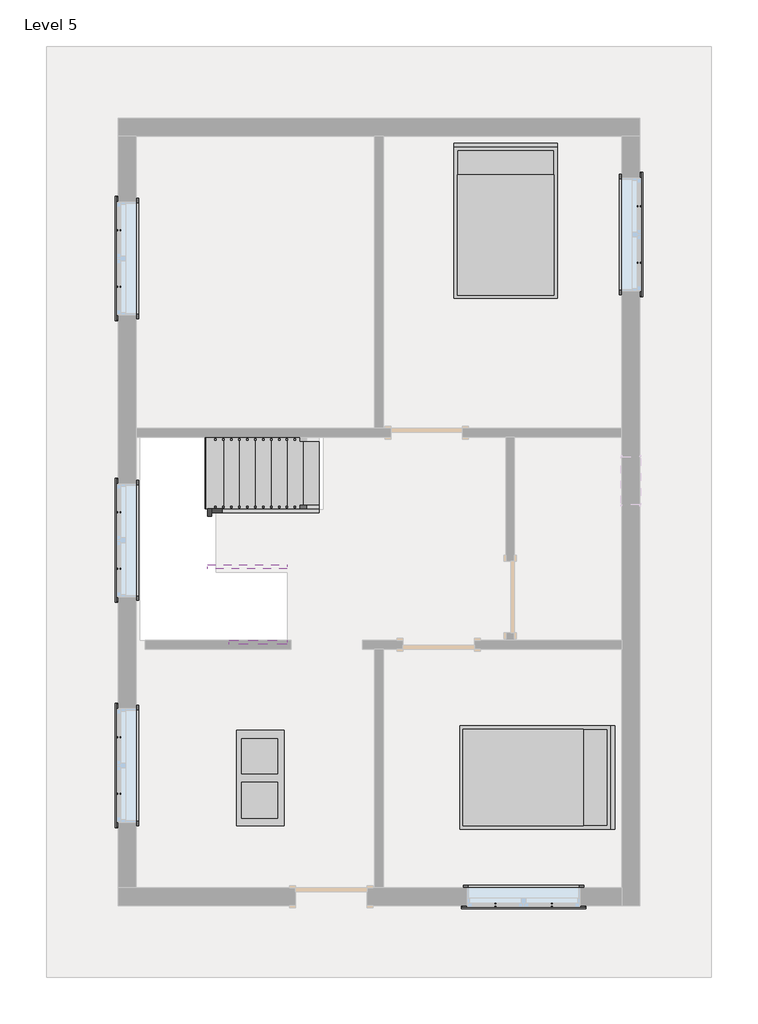
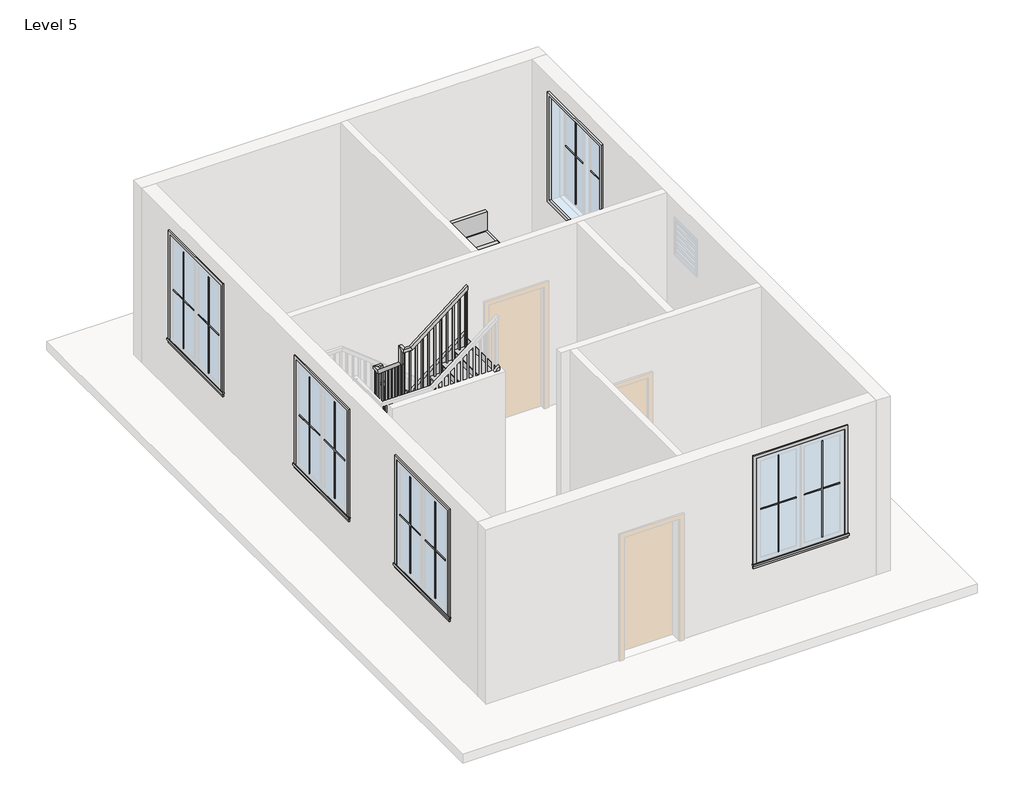
# One storey, part 2 of 2: 21 proxies, 5 members, 2 furniture elements, 1 railing, 1 stair flight.
"""IFC4 building model written with IfcOpenShell, lengths in millimetres."""

from ifc_helpers import new_model, si_unit, frame, origin, place, context, project, spatial, polyline, outline, extrude, faceted_brep, transform, mapped, element, save
from components import muntin_pattern_2x2_muntin_pattern_2x2_bff912c5, muntin_pattern_2x2_muntin_pattern_2x2_c2194282, trim_window_exterior_flat_with_sill_e04b3088, trim_window_interior_flat_picture_frame_2a7685fe, coffee_table_with_brass_mullions_11320_coffee_table_with_5962bef7, bed_17739_bed_17739_15c61121, stair_flight_03a67781

model = new_model("IFC4")

# Units and contexts
model_context = context("Model", 3, world=origin())
ifc_project = project(units=[si_unit("LENGTHUNIT", "METRE", prefix="MILLI")], contexts=[model_context])

# Site, building, storey
site = spatial("IfcSite", under=ifc_project)
building = spatial("IfcBuilding", under=site)
storey = spatial("IfcBuildingStorey", under=building, Name="Level 5", Elevation=9601.2)

# Proxies
placement = place(None, origin())
muntin_pattern_2x2_muntin_pattern_2x2_shape = muntin_pattern_2x2_muntin_pattern_2x2_bff912c5(model_context)
element("IfcBuildingElementProxy", 1, Name="Muntin Pattern_2x2 : Muntin Pattern_2x2", ObjectType="Muntin Pattern_2x2 : Muntin Pattern_2x2", at=placement, inside=storey, context=model_context, shape_type="MappedRepresentation", body=[
    mapped(muntin_pattern_2x2_muntin_pattern_2x2_shape, transform((-626.5715247, -5050.1430046, 10585.45), x_axis=(-1.0, 0.0, 0.0), y_axis=(0.0, -1.0, 0.0), z_axis=(0.0, 0.0, 1.0))),
])
element("IfcBuildingElementProxy", 2, Name="Muntin Pattern_2x2 : Muntin Pattern_2x2", ObjectType="Muntin Pattern_2x2 : Muntin Pattern_2x2", at=placement, inside=storey, context=model_context, shape_type="MappedRepresentation", body=[
    mapped(muntin_pattern_2x2_muntin_pattern_2x2_shape, transform((-6159.0090247, -3629.3305046, 10585.45), x_axis=(0.0, 1.0, 0.0), y_axis=(-1.0, 0.0, 0.0), z_axis=(0.0, 0.0, 1.0))),
])
element("IfcBuildingElementProxy", 3, Name="Muntin Pattern_2x2 : Muntin Pattern_2x2", ObjectType="Muntin Pattern_2x2 : Muntin Pattern_2x2", at=placement, inside=storey, context=model_context, shape_type="MappedRepresentation", body=[
    mapped(muntin_pattern_2x2_muntin_pattern_2x2_shape, transform((489.4409753, 3873.1944954, 10585.45), x_axis=(0.0, -1.0, 0.0), y_axis=(1.0, 0.0, 0.0), z_axis=(0.0, 0.0, 1.0))),
])
element("IfcBuildingElementProxy", 4, Name="Muntin Pattern_2x2 : Muntin Pattern_2x2", ObjectType="Muntin Pattern_2x2 : Muntin Pattern_2x2", at=placement, inside=storey, context=model_context, shape_type="MappedRepresentation", body=[
    mapped(muntin_pattern_2x2_muntin_pattern_2x2_shape, transform((-6159.0090247, 2847.6694954, 10585.45), x_axis=(0.0, 1.0, 0.0), y_axis=(-1.0, 0.0, 0.0), z_axis=(0.0, 0.0, 1.0))),
])
element("IfcBuildingElementProxy", 5, Name="Muntin Pattern_2x2 : Muntin Pattern_2x2", ObjectType="Muntin Pattern_2x2 : Muntin Pattern_2x2", at=placement, inside=storey, context=model_context, shape_type="MappedRepresentation", body=[
    mapped(muntin_pattern_2x2_muntin_pattern_2x2_shape, transform((-6159.0090247, -752.7805046, 10585.45), x_axis=(0.0, 1.0, 0.0), y_axis=(-1.0, 0.0, 0.0), z_axis=(0.0, 0.0, 1.0))),
])
muntin_pattern_2x2_muntin_pattern_2x2_2_shape = muntin_pattern_2x2_muntin_pattern_2x2_c2194282(model_context)
element("IfcBuildingElementProxy", 6, Name="Muntin Pattern_2x2 : Muntin Pattern_2x2", ObjectType="Muntin Pattern_2x2 : Muntin Pattern_2x2", at=placement, inside=storey, context=model_context, shape_type="MappedRepresentation", body=[
    mapped(muntin_pattern_2x2_muntin_pattern_2x2_2_shape, transform((-1347.2965247, -5050.1430046, 10585.45), x_axis=(1.0, 0.0, 0.0), y_axis=(0.0, 1.0, 0.0), z_axis=(0.0, 0.0, 1.0))),
])
element("IfcBuildingElementProxy", 7, Name="Muntin Pattern_2x2 : Muntin Pattern_2x2", ObjectType="Muntin Pattern_2x2 : Muntin Pattern_2x2", at=placement, inside=storey, context=model_context, shape_type="MappedRepresentation", body=[
    mapped(muntin_pattern_2x2_muntin_pattern_2x2_2_shape, transform((-6159.0090247, -2908.6055046, 10585.45), x_axis=(0.0, -1.0, 0.0), y_axis=(1.0, 0.0, 0.0), z_axis=(0.0, 0.0, 1.0))),
])
element("IfcBuildingElementProxy", 8, Name="Muntin Pattern_2x2 : Muntin Pattern_2x2", ObjectType="Muntin Pattern_2x2 : Muntin Pattern_2x2", at=placement, inside=storey, context=model_context, shape_type="MappedRepresentation", body=[
    mapped(muntin_pattern_2x2_muntin_pattern_2x2_2_shape, transform((489.4409753, 3152.4694954, 10585.45), x_axis=(0.0, 1.0, 0.0), y_axis=(-1.0, 0.0, 0.0), z_axis=(0.0, 0.0, 1.0))),
])
element("IfcBuildingElementProxy", 9, Name="Muntin Pattern_2x2 : Muntin Pattern_2x2", ObjectType="Muntin Pattern_2x2 : Muntin Pattern_2x2", at=placement, inside=storey, context=model_context, shape_type="MappedRepresentation", body=[
    mapped(muntin_pattern_2x2_muntin_pattern_2x2_2_shape, transform((-6159.0090247, 3568.3944954, 10585.45), x_axis=(0.0, -1.0, 0.0), y_axis=(1.0, 0.0, 0.0), z_axis=(0.0, 0.0, 1.0))),
])
element("IfcBuildingElementProxy", 10, Name="Muntin Pattern_2x2 : Muntin Pattern_2x2", ObjectType="Muntin Pattern_2x2 : Muntin Pattern_2x2", at=placement, inside=storey, context=model_context, shape_type="MappedRepresentation", body=[
    mapped(muntin_pattern_2x2_muntin_pattern_2x2_2_shape, transform((-6159.0090247, -32.0555046, 10585.45), x_axis=(0.0, -1.0, 0.0), y_axis=(1.0, 0.0, 0.0), z_axis=(0.0, 0.0, 1.0))),
])
trim_window_exterior_flat_with_sill_shape = trim_window_exterior_flat_with_sill_e04b3088(model_context)
element("IfcBuildingElementProxy", 11, Name="Trim-Window-Exterior-Flat : with Sill", ObjectType="Trim-Window-Exterior-Flat : with Sill", at=placement, inside=storey, context=model_context, shape_type="MappedRepresentation", body=[
    mapped(trim_window_exterior_flat_with_sill_shape, transform((-986.9340247, -5059.6680046, 12344.4), x_axis=(1.0, 0.0, 0.0), y_axis=(0.0, 0.0, 1.0), z_axis=(0.0, -1.0, 0.0))),
])
element("IfcBuildingElementProxy", 12, Name="Trim-Window-Exterior-Flat : with Sill", ObjectType="Trim-Window-Exterior-Flat : with Sill", at=placement, inside=storey, context=model_context, shape_type="MappedRepresentation", body=[
    mapped(trim_window_exterior_flat_with_sill_shape, transform((-6168.5340247, -3268.9680046, 12344.4), x_axis=(0.0, -1.0, 0.0), y_axis=(0.0, 0.0, 1.0), z_axis=(-1.0, 0.0, 0.0))),
])
element("IfcBuildingElementProxy", 13, Name="Trim-Window-Exterior-Flat : with Sill", ObjectType="Trim-Window-Exterior-Flat : with Sill", at=placement, inside=storey, context=model_context, shape_type="MappedRepresentation", body=[
    mapped(trim_window_exterior_flat_with_sill_shape, transform((498.9659753, 3512.8319954, 12344.4), x_axis=(0.0, 1.0, 0.0), y_axis=(0.0, 0.0, 1.0), z_axis=(1.0, 0.0, 0.0))),
])
element("IfcBuildingElementProxy", 14, Name="Trim-Window-Exterior-Flat : with Sill", ObjectType="Trim-Window-Exterior-Flat : with Sill", at=placement, inside=storey, context=model_context, shape_type="MappedRepresentation", body=[
    mapped(trim_window_exterior_flat_with_sill_shape, transform((-6168.5340247, 3208.0319954, 12344.4), x_axis=(0.0, -1.0, 0.0), y_axis=(0.0, 0.0, 1.0), z_axis=(-1.0, 0.0, 0.0))),
])
element("IfcBuildingElementProxy", 15, Name="Trim-Window-Exterior-Flat : with Sill", ObjectType="Trim-Window-Exterior-Flat : with Sill", at=placement, inside=storey, context=model_context, shape_type="MappedRepresentation", body=[
    mapped(trim_window_exterior_flat_with_sill_shape, transform((-6168.5340247, -392.4180046, 12344.4), x_axis=(0.0, -1.0, 0.0), y_axis=(0.0, 0.0, 1.0), z_axis=(-1.0, 0.0, 0.0))),
])
trim_window_interior_flat_picture_frame_shape = trim_window_interior_flat_picture_frame_2a7685fe(model_context)
element("IfcBuildingElementProxy", 16, Name="Trim-Window-Interior-Flat : Picture Frame", ObjectType="Trim-Window-Interior-Flat : Picture Frame", at=placement, inside=storey, context=model_context, shape_type="MappedRepresentation", body=[
    mapped(trim_window_interior_flat_picture_frame_shape, transform((-986.9340247, -4831.0680046, 12344.4), x_axis=(-1.0, 0.0, 0.0), y_axis=(0.0, 0.0, 1.0), z_axis=(0.0, 1.0, 0.0))),
])
element("IfcBuildingElementProxy", 17, Name="Trim-Window-Interior-Flat : Picture Frame", ObjectType="Trim-Window-Interior-Flat : Picture Frame", at=placement, inside=storey, context=model_context, shape_type="MappedRepresentation", body=[
    mapped(trim_window_interior_flat_picture_frame_shape, transform((-5939.9340247, -3268.9680046, 12344.4), x_axis=(0.0, 1.0, 0.0), y_axis=(0.0, 0.0, 1.0), z_axis=(1.0, 0.0, 0.0))),
])
element("IfcBuildingElementProxy", 18, Name="Trim-Window-Interior-Flat : Picture Frame", ObjectType="Trim-Window-Interior-Flat : Picture Frame", at=placement, inside=storey, context=model_context, shape_type="MappedRepresentation", body=[
    mapped(trim_window_interior_flat_picture_frame_shape, transform((270.3659753, 3512.8319954, 12344.4), x_axis=(0.0, -1.0, 0.0), y_axis=(0.0, 0.0, 1.0), z_axis=(-1.0, 0.0, 0.0))),
])
element("IfcBuildingElementProxy", 19, Name="Trim-Window-Interior-Flat : Picture Frame", ObjectType="Trim-Window-Interior-Flat : Picture Frame", at=placement, inside=storey, context=model_context, shape_type="MappedRepresentation", body=[
    mapped(trim_window_interior_flat_picture_frame_shape, transform((-5939.9340247, 3208.0319954, 12344.4), x_axis=(0.0, 1.0, 0.0), y_axis=(0.0, 0.0, 1.0), z_axis=(1.0, 0.0, 0.0))),
])
element("IfcBuildingElementProxy", 20, Name="Trim-Window-Interior-Flat : Picture Frame", ObjectType="Trim-Window-Interior-Flat : Picture Frame", at=placement, inside=storey, context=model_context, shape_type="MappedRepresentation", body=[
    mapped(trim_window_interior_flat_picture_frame_shape, transform((-5939.9340247, -392.4180046, 12344.4), x_axis=(0.0, 1.0, 0.0), y_axis=(0.0, 0.0, 1.0), z_axis=(1.0, 0.0, 0.0))),
])
coffee_table_with_brass_mullions_11320_coffee_table_with_shape = coffee_table_with_brass_mullions_11320_coffee_table_with_5962bef7(model_context)
element("IfcBuildingElementProxy", 21, Name="coffee_table_with_brass_mullions_11320 : coffee_table_with_brass_mullions_11320", ObjectType="coffee_table_with_brass_mullions_11320 : coffee_table_with_brass_mullions_11320", at=placement, inside=storey, context=model_context, shape_type="MappedRepresentation", body=[
    mapped(coffee_table_with_brass_mullions_11320_coffee_table_with_shape, transform((-3920.6340247, -2792.7180046, 9601.2), x_axis=(0.0, 1.0, 0.0), y_axis=(-1.0, 0.0, 0.0), z_axis=(0.0, 0.0, 1.0))),
])

# Furniture
bed_17739_bed_17739_shape = bed_17739_bed_17739_15c61121(model_context)
element("IfcFurniture", 22, ObjectType="Bed_17739 : Bed_17739", at=placement, inside=storey, context=model_context, shape_type="MappedRepresentation", body=[
    mapped(bed_17739_bed_17739_shape, transform((-1215.5340247, 3665.2319954, 9601.2), x_axis=(1.0, 0.0, 0.0), y_axis=(0.0, 1.0, 0.0), z_axis=(0.0, 0.0, 1.0))),
])
element("IfcFurniture", 23, ObjectType="Bed_17739 : Bed_17739", at=placement, inside=storey, context=model_context, shape_type="MappedRepresentation", body=[
    mapped(bed_17739_bed_17739_shape, transform((-834.5340247, -3421.3680046, 9601.2), x_axis=(0.0, -1.0, 0.0), y_axis=(1.0, 0.0, 0.0), z_axis=(0.0, 0.0, 1.0))),
])

# Members
element("IfcMember", 24, ObjectType="Stringer - 2\" Width", at=placement, inside=storey, context=model_context, shape_type="SweptSolid", body=[
    extrude(outline(polyline([(9601.2, -3603.1340247), (9832.7686588, -3603.1340247), (10915.6107641, -4974.7340247), (10527.2725136, -4974.7340247), (9601.2, -3801.7088408), (9601.2, -3603.1340247)])), frame((0.0, -43.1680046, 0.0), z_axis=(0.0, 1.0, 0.0), x_axis=(0.0, 0.0, 1.0)), (0.0, 0.0, 1.0), 50.8),
])
element("IfcMember", 25, ObjectType="Stringer - 2\" Width", at=placement, inside=storey, context=model_context, shape_type="SweptSolid", body=[
    extrude(outline(polyline([(7.6319954, 11122.4930346), (7.6319954, 10724.0154064), (-703.5680046, 11322.9206696), (-703.5680046, 11721.3982978), (7.6319954, 11122.4930346)])), frame((-5025.5340247, 0.0, 0.0), z_axis=(1.0, 0.0, 0.0), x_axis=(0.0, 1.0, 0.0)), (0.0, 0.0, 1.0), 50.8),
])
element("IfcMember", 26, ObjectType="Stringer - 2\" Width", at=placement, inside=storey, context=model_context, shape_type="SweptSolid", body=[
    extrude(outline(polyline([(11918.242343, -5025.5340247), (11529.9040926, -5025.5340247), (12332.0093557, -4009.5340247), (12720.3476062, -4009.5340247), (11918.242343, -5025.5340247)])), frame((0.0, -754.3680046, 0.0), z_axis=(0.0, 1.0, 0.0), x_axis=(0.0, 0.0, 1.0)), (0.0, 0.0, 1.0), 50.8),
])
element("IfcMember", 27, ObjectType="Stringer - 2\" Width", at=placement, inside=storey, context=model_context, shape_type="SweptSolid", body=[
    extrude(outline(polyline([(9601.2, -3603.1340247), (9832.7686588, -3603.1340247), (10352.471982, -4261.4249007), (10352.471982, -4753.3200179), (9601.2, -3801.7088408), (9601.2, -3603.1340247)])), frame((0.0, 922.0319954, 0.0), z_axis=(0.0, 1.0, 0.0), x_axis=(0.0, 0.0, 1.0)), (0.0, 0.0, 1.0), 50.8),
])
element("IfcMember", 28, ObjectType="Stringer - 2\" Width", at=placement, inside=storey, context=model_context, shape_type="SweptSolid", body=[
    extrude(outline(polyline([(12135.7206696, -4258.1663605), (12332.0093557, -4009.5340247), (12720.3476062, -4009.5340247), (12135.7206696, -4750.0614777), (12135.7206696, -4258.1663605)])), frame((0.0, -1719.5680046, 0.0), z_axis=(0.0, 1.0, 0.0), x_axis=(0.0, 0.0, 1.0)), (0.0, 0.0, 1.0), 50.8),
])

# Railing
element("IfcRailing", 29, ObjectType="Handrail - Rectangular", at=placement, inside=storey, context=model_context, shape_type="SolidModel", body=[
    faceted_brep([(-3603.1340247, 7.6319954, 10676.0210526), (-3603.1340247, 7.6319954, 10611.2980109), (-3603.1340247, 58.4319954, 10611.2980109), (-3603.1340247, 58.4319954, 10676.0210526), (-4949.3340247, 7.6319954, 11738.8105263), (-5000.1340247, 7.6319954, 11714.1927477), (-5000.1340247, 58.4319954, 11714.1927477), (-4949.3340247, 58.4319954, 11738.8105263), (-4949.3340247, 7.6319954, 12023.5578947), (-5000.1340247, 7.6319954, 11972.7578947), (-5000.1340247, 58.4319954, 11972.7578947), (-4949.3340247, 58.4319954, 12023.5578947), (-5025.5340247, 7.6319954, 12023.5578947), (-5025.5340247, 7.6319954, 11972.7578947), (-5076.3340247, 58.4319954, 11972.7578947), (-5076.3340247, 58.4319954, 12023.5578947), (-5025.5340247, -68.5680046, 12023.5578947), (-5025.5340247, -87.1083685, 11972.7578947), (-5076.3340247, -87.1083685, 11972.7578947), (-5076.3340247, -68.5680046, 12023.5578947), (-5025.5340247, -678.1680046, 12536.9052632), (-5025.5340247, -728.9680046, 12513.2712725), (-5076.3340247, -728.9680046, 12513.2712725), (-5076.3340247, -678.1680046, 12536.9052632), (-5025.5340247, -678.1680046, 12821.6526316), (-5025.5340247, -728.9680046, 12770.8526316), (-5076.3340247, -728.9680046, 12770.8526316), (-5076.3340247, -678.1680046, 12821.6526316), (-5025.5340247, -754.3680046, 12821.6526316), (-5025.5340247, -754.3680046, 12770.8526316), (-5076.3340247, -805.1680046, 12770.8526316), (-5076.3340247, -805.1680046, 12821.6526316), (-4949.3340247, -754.3680046, 12821.6526316), (-4931.6981718, -754.3680046, 12770.8526316), (-4931.6981718, -805.1680046, 12770.8526316), (-4949.3340247, -805.1680046, 12821.6526316), (-4009.5340247, -754.3680046, 13563.6), (-4009.5340247, -805.1680046, 13563.6), (-4009.5340247, -805.1680046, 13498.8769583), (-4009.5340247, -754.3680046, 13498.8769583)], [[[0, 1, 2, 3]], [[1, 0, 4, 5]], [[2, 1, 5, 6]], [[3, 2, 6, 7]], [[0, 3, 7, 4]], [[5, 4, 8, 9]], [[6, 5, 9, 10]], [[7, 6, 10, 11]], [[4, 7, 11, 8]], [[9, 8, 12, 13]], [[10, 9, 13, 14]], [[11, 10, 14, 15]], [[8, 11, 15, 12]], [[13, 12, 16, 17]], [[14, 13, 17, 18]], [[15, 14, 18, 19]], [[12, 15, 19, 16]], [[17, 16, 20, 21]], [[18, 17, 21, 22]], [[19, 18, 22, 23]], [[16, 19, 23, 20]], [[21, 20, 24, 25]], [[22, 21, 25, 26]], [[23, 22, 26, 27]], [[20, 23, 27, 24]], [[25, 24, 28, 29]], [[26, 25, 29, 30]], [[27, 26, 30, 31]], [[24, 27, 31, 28]], [[29, 28, 32, 33]], [[30, 29, 33, 34]], [[31, 30, 34, 35]], [[28, 31, 35, 32]], [[36, 37, 38, 39]], [[33, 32, 36, 39]], [[34, 33, 39, 38]], [[35, 34, 38, 37]], [[32, 35, 37, 36]]]),
    extrude(outline(polyline([(13471.3045898, -4044.4590247), (12488.7789474, -4044.4590247), (12488.7789474, -4025.4090247), (13486.3440635, -4025.4090247), (13471.3045898, -4044.4590247)])), frame((0.0, -789.2930046, 0.0), z_axis=(0.0, 1.0, 0.0), x_axis=(0.0, 0.0, 1.0)), (0.0, 0.0, 1.0), 19.05),
    extrude(outline(polyline([(13391.0940635, -4146.0590247), (12488.7789474, -4146.0590247), (12488.7789474, -4127.0090247), (13406.1335372, -4127.0090247), (13391.0940635, -4146.0590247)])), frame((0.0, -789.2930046, 0.0), z_axis=(0.0, 1.0, 0.0), x_axis=(0.0, 0.0, 1.0)), (0.0, 0.0, 1.0), 19.05),
    extrude(outline(polyline([(13310.8835372, -4247.6590247), (12328.3578947, -4247.6590247), (12328.3578947, -4228.6090247), (13325.9230109, -4228.6090247), (13310.8835372, -4247.6590247)])), frame((0.0, -789.2930046, 0.0), z_axis=(0.0, 1.0, 0.0), x_axis=(0.0, 0.0, 1.0)), (0.0, 0.0, 1.0), 19.05),
    extrude(outline(polyline([(13230.6730109, -4349.2590247), (12328.3578947, -4349.2590247), (12328.3578947, -4330.2090247), (13245.7124846, -4330.2090247), (13230.6730109, -4349.2590247)])), frame((0.0, -789.2930046, 0.0), z_axis=(0.0, 1.0, 0.0), x_axis=(0.0, 0.0, 1.0)), (0.0, 0.0, 1.0), 19.05),
    extrude(outline(polyline([(13150.4624846, -4450.8590247), (12167.9368421, -4450.8590247), (12167.9368421, -4431.8090247), (13165.5019583, -4431.8090247), (13150.4624846, -4450.8590247)])), frame((0.0, -789.2930046, 0.0), z_axis=(0.0, 1.0, 0.0), x_axis=(0.0, 0.0, 1.0)), (0.0, 0.0, 1.0), 19.05),
    extrude(outline(polyline([(13070.2519583, -4552.4590247), (12167.9368421, -4552.4590247), (12167.9368421, -4533.4090247), (13085.2914319, -4533.4090247), (13070.2519583, -4552.4590247)])), frame((0.0, -789.2930046, 0.0), z_axis=(0.0, 1.0, 0.0), x_axis=(0.0, 0.0, 1.0)), (0.0, 0.0, 1.0), 19.05),
    extrude(outline(polyline([(12990.0414319, -4654.0590247), (12007.5157895, -4654.0590247), (12007.5157895, -4635.0090247), (13005.0809056, -4635.0090247), (12990.0414319, -4654.0590247)])), frame((0.0, -789.2930046, 0.0), z_axis=(0.0, 1.0, 0.0), x_axis=(0.0, 0.0, 1.0)), (0.0, 0.0, 1.0), 19.05),
    extrude(outline(polyline([(12909.8309056, -4755.6590247), (12007.5157895, -4755.6590247), (12007.5157895, -4736.6090247), (12924.8703793, -4736.6090247), (12909.8309056, -4755.6590247)])), frame((0.0, -789.2930046, 0.0), z_axis=(0.0, 1.0, 0.0), x_axis=(0.0, 0.0, 1.0)), (0.0, 0.0, 1.0), 19.05),
    extrude(outline(polyline([(12829.6203793, -4857.2590247), (11847.0947368, -4857.2590247), (11847.0947368, -4838.2090247), (12844.659853, -4838.2090247), (12829.6203793, -4857.2590247)])), frame((0.0, -789.2930046, 0.0), z_axis=(0.0, 1.0, 0.0), x_axis=(0.0, 0.0, 1.0)), (0.0, 0.0, 1.0), 19.05),
    extrude(outline(polyline([(12749.409853, -4958.8590247), (11847.0947368, -4958.8590247), (11847.0947368, -4939.8090247), (12764.4493267, -4939.8090247), (12749.409853, -4958.8590247)])), frame((0.0, -789.2930046, 0.0), z_axis=(0.0, 1.0, 0.0), x_axis=(0.0, 0.0, 1.0)), (0.0, 0.0, 1.0), 19.05),
    extrude(outline(polyline([(-668.6430046, 12462.4712725), (-668.6430046, 11526.2526316), (-687.6930046, 11526.2526316), (-687.6930046, 12478.5133778), (-668.6430046, 12462.4712725)])), frame((-5060.4590247, 0.0, 0.0), z_axis=(1.0, 0.0, 0.0), x_axis=(0.0, 1.0, 0.0)), (0.0, 0.0, 1.0), 19.05),
    extrude(outline(polyline([(-567.0430046, 12376.9133778), (-567.0430046, 11526.2526316), (-586.0930046, 11526.2526316), (-586.0930046, 12392.955483), (-567.0430046, 12376.9133778)])), frame((-5060.4590247, 0.0, 0.0), z_axis=(1.0, 0.0, 0.0), x_axis=(0.0, 1.0, 0.0)), (0.0, 0.0, 1.0), 19.05),
    extrude(outline(polyline([(-465.4430046, 12291.355483), (-465.4430046, 11365.8315789), (-484.4930046, 11365.8315789), (-484.4930046, 12307.3975883), (-465.4430046, 12291.355483)])), frame((-5060.4590247, 0.0, 0.0), z_axis=(1.0, 0.0, 0.0), x_axis=(0.0, 1.0, 0.0)), (0.0, 0.0, 1.0), 19.05),
    extrude(outline(polyline([(-363.8430046, 12205.7975883), (-363.8430046, 11365.8315789), (-382.8930046, 11365.8315789), (-382.8930046, 12221.8396935), (-363.8430046, 12205.7975883)])), frame((-5060.4590247, 0.0, 0.0), z_axis=(1.0, 0.0, 0.0), x_axis=(0.0, 1.0, 0.0)), (0.0, 0.0, 1.0), 19.05),
    extrude(outline(polyline([(-262.2430046, 12120.2396935), (-262.2430046, 11205.4105263), (-281.2930046, 11205.4105263), (-281.2930046, 12136.2817988), (-262.2430046, 12120.2396935)])), frame((-5060.4590247, 0.0, 0.0), z_axis=(1.0, 0.0, 0.0), x_axis=(0.0, 1.0, 0.0)), (0.0, 0.0, 1.0), 19.05),
    extrude(outline(polyline([(-160.6430046, 12034.6817988), (-160.6430046, 11205.4105263), (-179.6930046, 11205.4105263), (-179.6930046, 12050.7239041), (-160.6430046, 12034.6817988)])), frame((-5060.4590247, 0.0, 0.0), z_axis=(1.0, 0.0, 0.0), x_axis=(0.0, 1.0, 0.0)), (0.0, 0.0, 1.0), 19.05),
    extrude(outline(polyline([(-59.0430046, 11949.1239041), (-59.0430046, 11044.9894737), (-78.0930046, 11044.9894737), (-78.0930046, 11965.1660093), (-59.0430046, 11949.1239041)])), frame((-5060.4590247, 0.0, 0.0), z_axis=(1.0, 0.0, 0.0), x_axis=(0.0, 1.0, 0.0)), (0.0, 0.0, 1.0), 19.05),
    extrude(outline(polyline([(-5016.0090247, 23.5069954), (-5035.0590247, 23.5069954), (-5035.0590247, 42.5569954), (-5016.0090247, 42.5569954), (-5016.0090247, 23.5069954)])), frame((0.0, 0.0, 10884.5684211), z_axis=(0.0, 0.0, 1.0), x_axis=(1.0, 0.0, 0.0)), (0.0, 0.0, 1.0), 1088.1894737),
    extrude(outline(polyline([(11661.5545898, -4933.4590247), (10724.1473684, -4933.4590247), (10724.1473684, -4914.4090247), (11646.5151161, -4914.4090247), (11661.5545898, -4933.4590247)])), frame((0.0, 23.5069954, 0.0), z_axis=(0.0, 1.0, 0.0), x_axis=(0.0, 0.0, 1.0)), (0.0, 0.0, 1.0), 19.05),
    extrude(outline(polyline([(11581.3440635, -4831.8590247), (10724.1473684, -4831.8590247), (10724.1473684, -4812.8090247), (11566.3045898, -4812.8090247), (11581.3440635, -4831.8590247)])), frame((0.0, 23.5069954, 0.0), z_axis=(0.0, 1.0, 0.0), x_axis=(0.0, 0.0, 1.0)), (0.0, 0.0, 1.0), 19.05),
    extrude(outline(polyline([(11501.1335372, -4730.2590247), (10563.7263158, -4730.2590247), (10563.7263158, -4711.2090247), (11486.0940635, -4711.2090247), (11501.1335372, -4730.2590247)])), frame((0.0, 23.5069954, 0.0), z_axis=(0.0, 1.0, 0.0), x_axis=(0.0, 0.0, 1.0)), (0.0, 0.0, 1.0), 19.05),
    extrude(outline(polyline([(11420.9230109, -4628.6590247), (10563.7263158, -4628.6590247), (10563.7263158, -4609.6090247), (11405.8835372, -4609.6090247), (11420.9230109, -4628.6590247)])), frame((0.0, 23.5069954, 0.0), z_axis=(0.0, 1.0, 0.0), x_axis=(0.0, 0.0, 1.0)), (0.0, 0.0, 1.0), 19.05),
    extrude(outline(polyline([(11340.7124846, -4527.0590247), (10403.3052632, -4527.0590247), (10403.3052632, -4508.0090247), (11325.6730109, -4508.0090247), (11340.7124846, -4527.0590247)])), frame((0.0, 23.5069954, 0.0), z_axis=(0.0, 1.0, 0.0), x_axis=(0.0, 0.0, 1.0)), (0.0, 0.0, 1.0), 19.05),
    extrude(outline(polyline([(11260.5019583, -4425.4590247), (10403.3052632, -4425.4590247), (10403.3052632, -4406.4090247), (11245.4624846, -4406.4090247), (11260.5019583, -4425.4590247)])), frame((0.0, 23.5069954, 0.0), z_axis=(0.0, 1.0, 0.0), x_axis=(0.0, 0.0, 1.0)), (0.0, 0.0, 1.0), 19.05),
    extrude(outline(polyline([(11180.2914319, -4323.8590247), (10242.8842105, -4323.8590247), (10242.8842105, -4304.8090247), (11165.2519583, -4304.8090247), (11180.2914319, -4323.8590247)])), frame((0.0, 23.5069954, 0.0), z_axis=(0.0, 1.0, 0.0), x_axis=(0.0, 0.0, 1.0)), (0.0, 0.0, 1.0), 19.05),
    extrude(outline(polyline([(11100.0809056, -4222.2590247), (10242.8842105, -4222.2590247), (10242.8842105, -4203.2090247), (11085.0414319, -4203.2090247), (11100.0809056, -4222.2590247)])), frame((0.0, 23.5069954, 0.0), z_axis=(0.0, 1.0, 0.0), x_axis=(0.0, 0.0, 1.0)), (0.0, 0.0, 1.0), 19.05),
    extrude(outline(polyline([(11019.8703793, -4120.6590247), (10082.4631579, -4120.6590247), (10082.4631579, -4101.6090247), (11004.8309056, -4101.6090247), (11019.8703793, -4120.6590247)])), frame((0.0, 23.5069954, 0.0), z_axis=(0.0, 1.0, 0.0), x_axis=(0.0, 0.0, 1.0)), (0.0, 0.0, 1.0), 19.05),
    extrude(outline(polyline([(10939.659853, -4019.0590247), (10082.4631579, -4019.0590247), (10082.4631579, -4000.0090247), (10924.6203793, -4000.0090247), (10939.659853, -4019.0590247)])), frame((0.0, 23.5069954, 0.0), z_axis=(0.0, 1.0, 0.0), x_axis=(0.0, 0.0, 1.0)), (0.0, 0.0, 1.0), 19.05),
    extrude(outline(polyline([(10859.4493267, -3917.4590247), (9922.0421053, -3917.4590247), (9922.0421053, -3898.4090247), (10844.409853, -3898.4090247), (10859.4493267, -3917.4590247)])), frame((0.0, 23.5069954, 0.0), z_axis=(0.0, 1.0, 0.0), x_axis=(0.0, 0.0, 1.0)), (0.0, 0.0, 1.0), 19.05),
    extrude(outline(polyline([(10779.2388004, -3815.8590247), (9922.0421053, -3815.8590247), (9922.0421053, -3796.8090247), (10764.1993267, -3796.8090247), (10779.2388004, -3815.8590247)])), frame((0.0, 23.5069954, 0.0), z_axis=(0.0, 1.0, 0.0), x_axis=(0.0, 0.0, 1.0)), (0.0, 0.0, 1.0), 19.05),
    extrude(outline(polyline([(10699.028274, -3714.2590247), (9761.6210526, -3714.2590247), (9761.6210526, -3695.2090247), (10683.9888004, -3695.2090247), (10699.028274, -3714.2590247)])), frame((0.0, 23.5069954, 0.0), z_axis=(0.0, 1.0, 0.0), x_axis=(0.0, 0.0, 1.0)), (0.0, 0.0, 1.0), 19.05),
    extrude(outline(polyline([(-5041.4090247, -770.2430046), (-5041.4090247, -789.2930046), (-5060.4590247, -789.2930046), (-5060.4590247, -770.2430046), (-5041.4090247, -770.2430046)])), frame((0.0, 0.0, 11686.6736842), z_axis=(0.0, 0.0, 1.0), x_axis=(1.0, 0.0, 0.0)), (0.0, 0.0, 1.0), 1084.1789474),
    extrude(outline(polyline([(-5041.4090247, 23.5069954), (-5060.4590247, 23.5069954), (-5060.4590247, 42.5569954), (-5041.4090247, 42.5569954), (-5041.4090247, 23.5069954)])), frame((0.0, 0.0, 10884.5684211), z_axis=(0.0, 0.0, 1.0), x_axis=(1.0, 0.0, 0.0)), (0.0, 0.0, 1.0), 1088.1894737),
    extrude(outline(polyline([(13483.8374846, -4028.5840247), (12488.7789474, -4028.5840247), (12488.7789474, -4009.5340247), (13498.8769583, -4009.5340247), (13483.8374846, -4028.5840247)])), frame((0.0, -789.2930046, 0.0), z_axis=(0.0, 1.0, 0.0), x_axis=(0.0, 0.0, 1.0)), (0.0, 0.0, 1.0), 19.05),
    extrude(outline(polyline([(10626.3374846, -3622.1840247), (9761.6210526, -3622.1840247), (9761.6210526, -3603.1340247), (10611.2980109, -3603.1340247), (10626.3374846, -3622.1840247)])), frame((0.0, 23.5069954, 0.0), z_axis=(0.0, 1.0, 0.0), x_axis=(0.0, 0.0, 1.0)), (0.0, 0.0, 1.0), 19.05),
])

# Stair flight
stair_flight_shape = stair_flight_03a67781(model_context)
element("IfcStairFlight", 30, ObjectType="2\" Tread 1\" Nosing 1/4\" Riser", at=placement, inside=storey, context=model_context, shape_type="MappedRepresentation", body=[
    mapped(stair_flight_shape, transform((0.0, 0.0, 0.0), x_axis=(1.0, 0.0, 0.0), y_axis=(0.0, 1.0, 0.0), z_axis=(0.0, 0.0, 1.0))),
])

save(model, "model.ifc")

# Revit data of these elements
# Type "Muntin Pattern_2x2 : Muntin Pattern_2x2"
#   Width [instance default] = 4' - 0"
#   Thickness = 0' - 0 1/2"
#   Height [instance default] = 4' - 0"
#   Distance = 0' - 0 3/4"
#   Interior Material [instance default] = none
#   Exterior Material [instance default] = none
#   Default Elevation = 0
# Type "Trim-Window-Exterior-Flat : with Sill"
#   Trim Width = 0' - 2 1/4"
#   Trim Thickness_Picture Frame = 0' - 1 1/4"
#   Trim Thickness_with Sill = 0' - 0 3/4"
#   Sill Thickness = 0' - 1 1/4"
#   Opening Width [instance default] = 2' - 0"
#   Opening Height [instance default] = 3' - 0"
#   Default Elevation = 4' - 0"
#   Sill = yes
#   Picture Frame = no
#   Trim Material [instance default] = none
# Type "Trim-Window-Interior-Flat : Picture Frame"
#   Trim Thickness_Picture Frame = 0' - 1 1/4"
#   Trim Width = 0' - 2 1/4"
#   Trim Thickness_with Sill = 0' - 0 3/4"
#   Sill Thickness = 0' - 1 1/4"
#   Opening Width [instance default] = 2' - 0"
#   Opening Height [instance default] = 3' - 0"
#   Default Elevation = 4' - 0"
#   Sill = no
#   Picture Frame = yes
#   Trim Material [instance default] = none
# Type "coffee_table_with_brass_mullions_11320 : coffee_table_with_brass_mullions_11320"
#   Default Elevation = 0
# Type "Bed_17739 : Bed_17739"
#   Default Elevation = 0
# Type "Handrail - Rectangular"
#   Assembly Code = "C2010400"
#   built-in parameter 1008612 = 0.0416667 (stored number, unit not read)
#   built-in parameter 1008611 = 0.0416667 (stored number, unit not read)
#   built-in parameter 1008609 = 0.333333 (stored number, unit not read)
#   built-in parameter 1008604 = 0.166667 (stored number, unit not read)
#   built-in parameter 1008603 = 0.166667 (stored number, unit not read)
#   Railing Height = 3' - 0"
#   built-in parameter 1008630 = 2
#   built-in parameter 1008610 = 2
#   built-in parameter 1008618 = Baluster - Square : 3/4"
# Elements 1, 2, 3, 4, 5, 6, 7, 8, 9, 10 (IfcBuildingElementProxy, "Muntin Pattern_2x2 : Muntin Pattern_2x2")
#   Width = 1' - 11 1/8"
#   Height = 5' - 6 1/2"
#   Interior Material = Wood - Stained
#   Exterior Material = Clad - White
#   Phase Created = New Construction
#   Materials on its faces: "Clad - White", "Wood - Stained"
# Elements 11, 12, 13, 14, 15 (IfcBuildingElementProxy, "Trim-Window-Exterior-Flat : with Sill")
#   Opening Width = 4' - 9"
#   Opening Height = 6' - 0"
#   Trim Material = Clad - White
#   Phase Created = New Construction
#   Materials on its faces: "Clad - White"
# Elements 16, 17, 18, 19, 20 (IfcBuildingElementProxy, "Trim-Window-Interior-Flat : Picture Frame")
#   Opening Width = 4' - 9"
#   Opening Height = 6' - 0"
#   Trim Material = Wood - Stained
#   Phase Created = New Construction
#   Materials on its faces: "Wood - Stained"
# Element 21 (IfcBuildingElementProxy, "coffee_table_with_brass_mullions_11320 : coffee_table_with_brass_mullions_11320")
#   Phase Created = New Construction
#   Materials on its faces: "Default Wall", "TABLE", "Glass", "Default"
# Elements 22, 23 (IfcFurniture, "Bed_17739 : Bed_17739")
#   Phase Created = New Construction
#   Materials on its faces: "legs", "sheets", "bed frame", "Blanket"
# Elements 24, 25, 26, 27, 28 (IfcMember, "Stringer - 2\" Width")
#   Phase Created = New Construction
# Element 29 (IfcRailing, "Handrail - Rectangular")
#   Phase Created = New Construction
#   Materials on its faces: "Oak Flooring"
# Element 30 (IfcStairFlight, "2\" Tread 1\" Nosing 1/4\" Riser")
#   Phase Created = New Construction
# Materials
#   "Clad - White": class "Wood", colour RGB 242 242 238, transparency 0, Cost = 0
#   "Wood - Stained": class "Wood", colour RGB 224 178 126, transparency 0, Cost = 0
#   "Default Wall": colour RGB 128 128 128, transparency 0, Cost = 0
#   "TABLE": class "Generic", colour RGB 120 120 120, transparency 0, Cost = 0
#   "Glass": class "Glass", colour RGB 0 128 192, transparency 0.75, Description = "Soda Lime Glass", Cost = 0
#   "Default": colour RGB 127 127 127, transparency 0, Cost = 0
#   "legs": colour RGB 90 73 37, transparency 0, Cost = 0
#   "sheets": colour RGB 200 195 176, transparency 0, Cost = 0
#   "bed frame": colour RGB 90 73 37, transparency 0, Cost = 0
#   "Blanket": class "System", colour RGB 59 0 1, transparency 0, Cost = 0
#   "Oak Flooring": class "Wood", colour RGB 216 169 114, transparency 0, Description = "Quercus Rubra", Cost = 0
